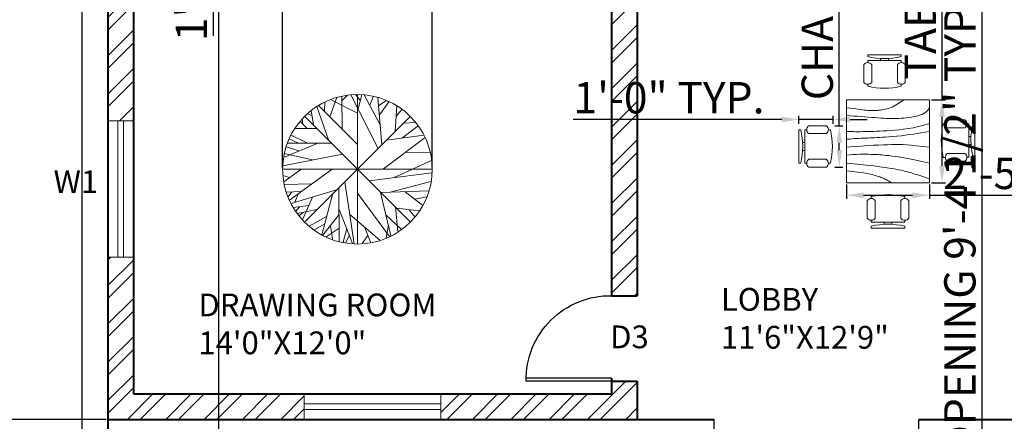
# Model space of a CAD drawing. Units: inches. Extents: x 2069 to 3028, y 691 to 1726.
# Tile 3 of 10: x 2267 to 2613, y 903 to 1044. Entities that reach past the tile are written whole.
import ezdxf

# ---------------------------------------------------------------- set-up
doc = ezdxf.new("R2010")
doc.units = ezdxf.units.IN
for name, color, linetype, lineweight in [('A-ANNO-DIMS', 2, 'Continuous', 18), ('A-DOOR', 3, 'Continuous', 25), ('A-FLOR', 7, 'Continuous', 25), ('A-FURN', 8, 'Continuous', 18), ('A-GLAZ', 4, 'Continuous', 20), ('A-WALL', 7, 'Continuous', 40)]:
    doc.layers.add(name, color=color, linetype=linetype, lineweight=lineweight)
for name, color, linetype, lineweight, true_color in [('A-ANNO-TEXT', 11, 'Continuous', 18, 0xf27172), ('A-AREA-IDEN', 11, 'Continuous', 25, 0xf27172), ('A-WALL-PATT', 143, 'Continuous', 13, 0x7aafdf), ('L-PLNT', 2, 'Continuous', 13, 0xf1eb1f)]:
    doc.layers.add(name, color=color, linetype=linetype, lineweight=lineweight, true_color=true_color)
doc.styles.get("Standard").update_dxf_attribs({"font": 'arial.ttf'})
doc.dimstyles.new('ISO-25', dxfattribs={"dimtxt": 11, "dimasz": 6, "dimexe": 1.25, "dimexo": 0.625, "dimtad": 1, "dimlunit": 3, "dimtxsty": 'Standard', "dimcen": 2.5, "dimclrd": 3, "dimclre": 5, "dimclrt": 6, "dimadec": 0, "dimazin": 0, "dimtfac": 1, "dimtmove": 0, "dimatfit": 3, "dimfxl": 1, "dimarcsym": 0})

# ---------------------------------------------------------------- blocks, each defined once
blk = doc.blocks.new('Table - Square Woodgrain 42 x 42 in.')
blk.add_line((0, -42), (42, -42))
for points in [[(0, -4), (1.704, -4.2172), (3.2358, -4.4188), (4.615, -4.604), (5.8615, -4.7721), (6.9951, -4.9224), (8.0357, -5.0541), (9.0031, -5.1667), (9.9171, -5.2594), (10.7951, -5.3316), (11.6445, -5.3836), (12.4702, -5.4157), (13.277, -5.4283), (14.0698, -5.4217), (14.8535, -5.3964), (15.6331, -5.3526), (16.4133, -5.2908), (17.1986, -5.2103), (17.9913, -5.1062), (18.793, -4.9727), (19.6056, -4.8038), (20.4307, -4.5937), (21.2701, -4.3365), (22.1256, -4.0262), (22.9989, -3.6571), (23.888, -3.2272), (24.7756, -2.7516), (25.6408, -2.2491), (26.4624, -1.7387), (27.2195, -1.2395), (27.891, -0.7703), (28.456, -0.3501), (28.8934, 0.002)], [(0, -42), (0, 0), (42, 0), (42, -42)], [(0, -8), (1.8203, -8.1001), (3.6741, -8.2149), (5.5411, -8.3408), (7.4011, -8.4741), (9.2339, -8.6112), (11.0193, -8.7484), (12.7371, -8.8821), (14.3671, -9.0086), (15.8954, -9.1246), (17.3337, -9.2278), (18.6997, -9.3159), (20.0116, -9.387), (21.2871, -9.4389), (22.5442, -9.4696), (23.8008, -9.477), (25.0749, -9.459), (26.3791, -9.4137), (27.7049, -9.3403), (29.0383, -9.2382), (30.3655, -9.1068), (31.6728, -8.9455), (32.9461, -8.7535), (34.1717, -8.5304), (35.3358, -8.2756), (36.4268, -7.9863), (37.443, -7.6521), (38.3849, -7.2603), (39.253, -6.7986), (40.048, -6.2542), (40.7705, -5.6147), (41.421, -4.8674), (42, -4)], [(42, -12), (39.1784, -12.8621), (36.4519, -13.5654), (33.8246, -14.1294), (31.3004, -14.5731), (28.8832, -14.9161), (26.577, -15.1775), (24.3858, -15.3768), (22.3136, -15.5332), (20.3622, -15.6632), (18.5254, -15.7718), (16.7947, -15.8612), (15.1618, -15.9338), (13.6183, -15.9916), (12.1558, -16.0369), (10.7659, -16.0718), (9.4403, -16.0987), (8.1703, -16.1191), (6.9461, -16.1325), (5.7577, -16.1377), (4.595, -16.1335), (3.4479, -16.1188), (2.3064, -16.0924), (1.1604, -16.0532), (0, -16)], [(42, -16), (37.6529, -16.7365), (33.8802, -17.329), (30.6179, -17.7961), (27.8015, -18.1561), (25.3668, -18.4275), (23.2497, -18.6288), (21.3859, -18.7785), (19.7111, -18.8949), (18.1693, -18.9939), (16.7375, -19.0795), (15.401, -19.1534), (14.1449, -19.217), (12.9544, -19.2717), (11.8148, -19.3191), (10.7113, -19.3606), (9.6291, -19.3976), (8.5534, -19.4323), (7.47, -19.4689), (6.3643, -19.5122), (5.222, -19.5672), (4.0288, -19.6386), (2.7703, -19.7313), (1.4321, -19.8501), (0, -20)], [(0, -24), (3.9243, -23.6805), (7.4766, -23.4138), (10.6891, -23.1954), (13.5943, -23.0205), (16.2247, -22.8847), (18.6125, -22.7832), (20.7903, -22.7116), (22.7903, -22.6651), (24.6563, -22.642), (26.4764, -22.6507), (28.35, -22.7024), (30.3766, -22.8084), (32.6555, -22.98), (35.2861, -23.2283), (38.3678, -23.5645), (42, -24)], [(42, -32), (37.392, -31.017), (33.4585, -30.2231), (30.1291, -29.5949), (27.3334, -29.109), (25.0009, -28.742), (23.0612, -28.4707), (21.4439, -28.2716), (20.0786, -28.1215), (18.8998, -28.0002), (17.8609, -27.9014), (16.9206, -27.8219), (16.0371, -27.7588), (15.1691, -27.709), (14.2748, -27.6693), (13.3128, -27.6368), (12.2415, -27.6083), (11.0295, -27.5824), (9.6867, -27.5643), (8.233, -27.5608), (6.6884, -27.5787), (5.0728, -27.6248), (3.4062, -27.7058), (1.7086, -27.8286), (0, -28)], [(0, -32), (5.4026, -32.5358), (9.9494, -33.019), (13.7424, -33.4553), (16.8834, -33.8505), (19.4743, -34.2106), (21.6171, -34.5413), (23.4136, -34.8486), (24.9657, -35.1382), (26.3614, -35.4156), (27.6332, -35.6841), (28.7995, -35.9467), (29.8788, -36.2064), (30.8897, -36.4661), (31.8507, -36.7288), (32.7802, -36.9973), (33.6968, -37.2747), (34.6175, -37.5635), (35.5531, -37.8651), (36.5128, -38.1805), (37.506, -38.5108), (38.5421, -38.8568), (39.6302, -39.2197), (40.7797, -39.6004), (42, -40)], [(0, -36), (3.0098, -36.2857), (5.5354, -36.5643), (7.6368, -36.8359), (9.374, -37.1009), (10.807, -37.3597), (11.9957, -37.6126), (13.0002, -37.8599), (13.8804, -38.102), (14.6874, -38.3393), (15.4365, -38.5729), (16.1338, -38.8041), (16.7858, -39.0341), (17.3987, -39.264), (17.9787, -39.4952), (18.5322, -39.7288), (19.0655, -39.9662), (19.5832, -40.2081), (20.0842, -40.4544), (20.5657, -40.7046), (21.0249, -40.9581), (21.459, -41.2144), (21.8653, -41.4731), (22.2409, -41.7335), (22.5831, -41.9951)]]:
    blk.add_lwpolyline(points)
blk = doc.blocks.new('Chair - Desk')
for p, q in [((-8.5, 0), (-8.5, -1)), ((-8.5, 0), (8.5, 0)), ((8.5, 0), (8.5, -1)), ((-8.5, -3), (-8.5, -4)), ((-8.5, -3), (8.5, -3)), ((-2, -3), (-2, -1.9355)), ((2, -1.9576), (2, -3)), ((8.5, -3), (8.5, -4)), ((-10.5, -5), (-10.5, -14)), ((-6.5, -14), (-6.5, -5)), ((6.5, -5), (6.5, -14)), ((10.5, -14), (10.5, -5)), ((-8.5, -15), (-8.5, -16)), ((8.5, -15), (8.5, -16))]:
    blk.add_line(p, q)
for centre, radius, start, end in [((-8.5, -6.5), 2.5, 36.8699, 143.1301), ((0, 34.625), 36.625, 256.5803, 283.4197), ((8.5, -6.5), 2.5, 36.8699, 143.1301), ((-8.5, -12.5), 2.5, 216.8699, 323.1301), ((8.5, -12.5), 2.5, 216.8699, 323.1301), ((0, 19.625), 36.625, 256.5803, 283.4197)]:
    blk.add_arc(centre, radius, start, end)
blk = doc.blocks.new('*U15')
for p, q in [((-559.96332, 1068.71262), (-421.33774, 1464.27444)), ((-537.60624, 1418.42744), (-0.98552, 1143.23876)), ((-318.48552, 1395.49124), (-202.21702, 1510.14684)), ((-314.01258, 816.46522), (-318.48552, 1492.95104)), ((-135.1407, 1515.88724), (419.3667, 426.62602)), ((61.6204, 1395.49124), (-36.75888, 1521.60224)), ((0, 1523.98984), (0, -1524)), ((12.43076, 1234.96832), (92.92336, 1515.88724)), ((464.08594, 902.45692), (137.6426, 1515.88724)), ((249.43562, 1309.49446), (325.45782, 1487.21064)), ((499.8593, 495.41938), (414.89376, 1464.27444)), ((-828.27368, 1280.83056), (-591.26628, 598.61196)), ((-792.50032, 1298.0289), (-5.45846, 512.61772)), ((-671.75888, 1183.37076), (-667.28848, 1366.81464)), ((432.78298, 1298.0289), (589.29524, 1401.23164)), ((450.66966, 1108.84208), (647.43076, 1378.29544)), ((803.94302, 1292.29612), (768.16966, 776.33322)), ((790.52928, 1080.17818), (911.26818, 1223.50022)), ((-1114.47072, 925.38804), (-1127.887, 1022.84784)), ((1066.8, 1066.8), (-1066.8, -1066.8)), ((1066.8, -1066.8), (-1066.8, 1066.8)), ((-1020.56438, 1131.7732), (-926.6555, 1097.37652)), ((-940.07178, 1194.83632), (-895.35, 902.45692)), ((-1266.51258, 833.66356), (-832.74662, 833.66356)), ((-1163.66036, 971.25282), (-1029.50772, 839.39634)), ((920.21152, 638.74396), (1242.18446, 890.99136)), ((942.57114, 942.58892), (1184.04894, 954.05448)), ((-1391.72442, 621.54308), (-1212.85, 535.55138)), ((-1351.47812, 696.07176), (-1020.56438, 529.8186)), ((1380.81004, 644.47674), (531.16226, 8.12292)), ((593.76818, 592.87918), (1353.98002, 696.07176)), ((-819.33034, 524.08582), (-1503.51998, 237.4392)), ((-1449.8574, 455.28992), (-1194.96332, 375.02846)), ((-1423.02738, 529.8186), (-528.66036, 529.8186)), ((-1516.93626, 71.1835), (-305.06924, 306.2351)), ((-1490.10624, 323.43344), (-913.23922, 191.57696)), ((978.3445, 340.63178), (1479.19186, 346.36456)), ((-1387.25148, -628.2309), (-515.24662, 2.39014)), ((745.81004, -169.59834), (1510.49228, 180.1114)), ((-1524, 0), (1524, 0)), ((-1516.93626, -123.73356), (-1378.30814, -169.59834)), ((-1150.24662, -3.34264), (-1499.04958, -255.59258)), ((236.02188, -232.65892), (1514.96522, -72.13854)), ((-1485.6333, -312.92038), (-926.6555, -295.72204)), ((-376.6185, -381.71628), (-372.1481, -1465.2371)), ((-255.8796, -255.59258), (-63.59144, -1516.83212)), ((669.79038, -467.71052), (1497.07854, -249.85726)), ((-1449.8574, -467.71052), (-1150.24662, -456.24496)), ((-1338.06438, -461.9752), (-1409.61364, -559.43754)), ((-1351.47812, -697.0268), (-425.80814, -421.84574)), ((-1199.43626, -490.64164), (-1275.45592, -668.3629)), ((-913.23922, -570.9031), (-1118.94366, -1029.53566)), ((-506.30074, -513.57276), (-725.42146, -1339.1134)), ((-0.98552, -484.90886), (656.3741, -1367.7773)), ((473.02928, -473.44076), (678.73372, -1356.31174)), ((477.49968, -473.44076), (1456.83224, -439.04662)), ((969.40116, -461.9752), (1331.6204, -737.15626)), ((1166.16226, -611.03256), (1412.113, -565.17032)), ((-989.25888, -737.15626), (-1306.75888, -777.28572)), ((-1181.54958, -765.82016), (-1257.56924, -851.8144)), ((772.6426, -765.82016), (821.83224, -1270.3175)), ((799.47262, -794.4866), (1260.07114, -846.08162)), ((-823.80074, -823.1505), (-1221.79334, -903.41196)), ((-1110.00032, -880.4783), (-1186.01998, -949.2742)), ((-627.04218, -960.73976), (-984.78848, -1161.39214)), ((-372.1481, -920.6103), (-703.06438, -1344.84618)), ((-372.1481, -817.41772), (-99.3648, -1511.10188)), ((-157.50032, -920.6103), (455.1426, -1448.03876)), ((580.3519, -926.34308), (897.8519, -1230.18804)), ((1054.3667, -828.88328), (1170.6352, -966.47254)), ((-667.28848, -1115.5299), (-881.93626, -1235.92082)), ((-372.1481, -1201.52414), (-635.98552, -1379.24286)), ((-546.54958, -1155.65936), (-506.30074, -1425.1051)), ((151.05634, -1184.32326), (267.32484, -1488.16822)), ((629.54408, -1138.46102), (584.82484, -1396.4412)), ((-215.6333, -1207.25692), (-291.6555, -1488.16822)), ((-161.97072, -1339.1134), (-237.99292, -1493.901)), ((213.66226, -1350.57896), (97.39376, -1511.10188))]:
    blk.add_line(p, q)
blk.add_circle((0, 0), 1524)
blk = doc.blocks.new('DOOR-SWING-30IN')
for p, q in [((-1, 0), (-1, 30)), ((0, 0), (0, 30))]:
    blk.add_line(p, q)
blk.add_arc((-0.5, 0.5), 29.5, 89.029, 180.971)
blk = doc.blocks.new('WINDOW-SASH-48IN')
for p, q in [((0, 0), (48, 0)), ((0, -2), (48, -2))]:
    blk.add_line(p, q)
blk = doc.blocks.new('*D46')
at = {"layer": 'A-ANNO-DIMS', "color": 3, "lineweight": -2, "transparency": 16777216}
for p, q in [((2554.97, 1007.13), (2554.97, 1159.02)), ((2554.97, 998.55), (2554.97, 1001.13))]:
    blk.add_line(p, q, dxfattribs=at)
at = {"layer": 'A-ANNO-DIMS', "color": 5, "lineweight": -2, "transparency": 16777216}
for p, q in [((2553.4, 1007.13), (2556.22, 1007.13)), ((2553.4, 992.55), (2556.22, 992.55))]:
    blk.add_line(p, q, dxfattribs=at)
at = {"layer": 'A-ANNO-DIMS', "color": 3, "transparency": 16777216}
for points in [[(2553.97, 1001.13), (2555.97, 1001.13), (2554.97, 1007.13)], [(2553.97, 998.55), (2555.97, 998.55), (2554.97, 992.55)]]:
    blk.add_solid(points, dxfattribs=at)
at = {"layer": 'Defpoints', "color": 0, "transparency": 16777216}
for p in [(2552.78, 1007.13), (2554.97, 1007.13), (2552.78, 992.55)]:
    blk.add_point(p, dxfattribs=at)
at = {"layer": 'A-ANNO-DIMS', "color": 6, "transparency": 16777216, "insert": (2548.65, 1086.08), "char_height": 11, "attachment_point": 5, "rotation": 90}
blk.add_mtext('CHAIR 1\'-2 1/2" TYP.', dxfattribs=at)
blk = doc.blocks.new('*D47')
at = {"layer": 'A-ANNO-DIMS', "color": 5, "lineweight": -2, "transparency": 16777216}
for p, q in [((2540.74, 1007.76), (2540.74, 1010.57)), ((2552.78, 1007.76), (2552.78, 1010.57))]:
    blk.add_line(p, q, dxfattribs=at)
at = {"layer": 'A-ANNO-DIMS', "color": 3, "lineweight": -2, "transparency": 16777216}
for p, q in [((2534.74, 1009.32), (2461.47, 1009.32)), ((2552.78, 1009.32), (2540.74, 1009.32)), ((2558.78, 1009.32), (2564.78, 1009.32))]:
    blk.add_line(p, q, dxfattribs=at)
at = {"layer": 'A-ANNO-DIMS', "color": 3, "transparency": 16777216}
for points in [[(2534.74, 1010.32), (2534.74, 1008.32), (2540.74, 1009.32)], [(2558.78, 1010.32), (2558.78, 1008.32), (2552.78, 1009.32)]]:
    blk.add_solid(points, dxfattribs=at)
at = {"layer": 'Defpoints', "color": 0, "transparency": 16777216}
for p in [(2540.74, 1009.32), (2540.74, 1007.13), (2552.78, 1007.13)]:
    blk.add_point(p, dxfattribs=at)
at = {"layer": 'A-ANNO-DIMS', "color": 6, "transparency": 16777216, "insert": (2495.11, 1015.56), "char_height": 11, "attachment_point": 5}
blk.add_mtext('1\'-0" TYP.', dxfattribs=at)
blk = doc.blocks.new('*D66')
at = {"layer": 'A-ANNO-DIMS', "color": 3, "lineweight": -2, "transparency": 16777216}
for p, q in [((2591.06, 1016.25), (2591.06, 1105.97)), ((2591.06, 993.08), (2591.06, 1010.25))]:
    blk.add_line(p, q, dxfattribs=at)
at = {"layer": 'A-ANNO-DIMS', "color": 5, "lineweight": -2, "transparency": 16777216}
for p, q in [((2587.31, 1016.25), (2592.31, 1016.25)), ((2587.31, 987.08), (2592.31, 987.08))]:
    blk.add_line(p, q, dxfattribs=at)
at = {"layer": 'A-ANNO-DIMS', "color": 3, "transparency": 16777216}
for points in [[(2590.06, 1010.25), (2592.06, 1010.25), (2591.06, 1016.25)], [(2590.06, 993.08), (2592.06, 993.08), (2591.06, 987.08)]]:
    blk.add_solid(points, dxfattribs=at)
at = {"layer": 'Defpoints', "color": 0, "transparency": 16777216}
for p in [(2586.69, 1016.25), (2591.06, 1016.25), (2586.69, 987.08)]:
    blk.add_point(p, dxfattribs=at)
at = {"layer": 'A-ANNO-DIMS', "color": 6, "transparency": 16777216, "insert": (2584.82, 1064.11), "char_height": 11, "attachment_point": 5, "rotation": 90}
blk.add_mtext('TABLE 2\'-5"', dxfattribs=at)
blk = doc.blocks.new('*D67')
at = {"layer": 'A-ANNO-DIMS', "color": 5, "lineweight": -2, "transparency": 16777216}
for p, q in [((2557.52, 986.45), (2557.52, 981.45)), ((2586.69, 986.45), (2586.69, 981.45))]:
    blk.add_line(p, q, dxfattribs=at)
at = {"layer": 'A-ANNO-DIMS', "color": 3, "lineweight": -2, "transparency": 16777216}
for p, q in [((2563.52, 982.7), (2580.69, 982.7)), ((2586.69, 982.7), (2623.36, 982.7))]:
    blk.add_line(p, q, dxfattribs=at)
at = {"layer": 'A-ANNO-DIMS', "color": 3, "transparency": 16777216}
for points in [[(2563.52, 983.7), (2563.52, 981.7), (2557.52, 982.7)], [(2580.69, 983.7), (2580.69, 981.7), (2586.69, 982.7)]]:
    blk.add_solid(points, dxfattribs=at)
at = {"layer": 'Defpoints', "color": 0, "transparency": 16777216}
for p in [(2557.52, 987.08), (2586.69, 987.08), (2586.69, 982.7)]:
    blk.add_point(p, dxfattribs=at)
at = {"layer": 'A-ANNO-DIMS', "color": 6, "transparency": 16777216, "insert": (2608.03, 988.95), "char_height": 11, "attachment_point": 5}
blk.add_mtext('2\'-5"', dxfattribs=at)
blk = doc.blocks.new('*D72')
at = {"layer": 'A-ANNO-DIMS', "color": 5, "lineweight": -2, "transparency": 16777216}
for p, q in [((2621.33, 1178.39), (2603.83, 1178.39)), ((2621.33, 1065.89), (2603.83, 1065.89))]:
    blk.add_line(p, q, dxfattribs=at)
at = {"layer": 'A-ANNO-DIMS', "color": 3, "lineweight": -2, "transparency": 16777216}
for p, q in [((2605.08, 1172.39), (2605.08, 1071.89)), ((2605.08, 1065.89), (2605.08, 833.73))]:
    blk.add_line(p, q, dxfattribs=at)
at = {"layer": 'A-ANNO-DIMS', "color": 3, "transparency": 16777216}
for points in [[(2604.08, 1172.39), (2606.08, 1172.39), (2605.08, 1178.39)], [(2604.08, 1071.89), (2606.08, 1071.89), (2605.08, 1065.89)]]:
    blk.add_solid(points, dxfattribs=at)
at = {"layer": 'Defpoints', "color": 0, "transparency": 16777216}
for p in [(2621.95, 1178.39), (2605.08, 1065.89), (2621.95, 1065.89)]:
    blk.add_point(p, dxfattribs=at)
at = {"layer": 'A-ANNO-DIMS', "color": 6, "transparency": 16777216, "insert": (2598.76, 946.81), "char_height": 11, "attachment_point": 5, "rotation": 90}
blk.add_mtext('CASED OPENING 9\'-4 1/2" TYP.', dxfattribs=at)
blk = doc.blocks.new('*D85')
at = {"layer": 'A-ANNO-DIMS', "color": 5, "lineweight": -2, "transparency": 16777216}
for p, q in [((2339.28, 1095.19), (2333.7, 1095.19)), ((2339.28, 1074.19), (2333.7, 1074.19))]:
    blk.add_line(p, q, dxfattribs=at)
at = {"layer": 'A-ANNO-DIMS', "color": 3, "lineweight": -2, "transparency": 16777216}
for p, q in [((2334.95, 1089.19), (2334.95, 1080.19)), ((2334.95, 1074.19), (2334.95, 1038.73))]:
    blk.add_line(p, q, dxfattribs=at)
at = {"layer": 'A-ANNO-DIMS', "color": 3, "transparency": 16777216}
for points in [[(2333.95, 1089.19), (2335.95, 1089.19), (2334.95, 1095.19)], [(2333.95, 1080.19), (2335.95, 1080.19), (2334.95, 1074.19)]]:
    blk.add_solid(points, dxfattribs=at)
at = {"layer": 'Defpoints', "color": 0, "transparency": 16777216}
for p in [(2339.91, 1095.19), (2334.95, 1074.19), (2339.91, 1074.19)]:
    blk.add_point(p, dxfattribs=at)
at = {"layer": 'A-ANNO-DIMS', "color": 6, "transparency": 16777216, "insert": (2328.71, 1053.46), "char_height": 11, "attachment_point": 5, "rotation": 90}
blk.add_mtext('1\'-9"', dxfattribs=at)
blk = doc.blocks.new('*D87')
at = {"layer": 'A-ANNO-DIMS', "color": 5, "lineweight": -2, "transparency": 16777216}
for p, q in [((2297.33, 1487.39), (2090.2, 1487.39)), ((2297.33, 903.89), (2090.2, 903.89))]:
    blk.add_line(p, q, dxfattribs=at)
at = {"layer": 'A-ANNO-DIMS', "color": 3, "lineweight": -2, "transparency": 16777216}
blk.add_line((2091.45, 909.89), (2091.45, 1481.39), dxfattribs=at)
at = {"layer": 'A-ANNO-DIMS', "color": 3, "transparency": 16777216}
for points in [[(2090.45, 1481.39), (2092.45, 1481.39), (2091.45, 1487.39)], [(2090.45, 909.89), (2092.45, 909.89), (2091.45, 903.89)]]:
    blk.add_solid(points, dxfattribs=at)
at = {"layer": 'Defpoints', "color": 0, "transparency": 16777216}
for p in [(2091.45, 1487.39), (2297.95, 1487.39), (2297.95, 903.89)]:
    blk.add_point(p, dxfattribs=at)
at = {"layer": 'A-ANNO-DIMS', "color": 6, "transparency": 16777216, "insert": (2085.14, 1195.64), "char_height": 11, "attachment_point": 5, "rotation": 90}
blk.add_mtext('48\'-7 1/2"', dxfattribs=at)
blk = doc.blocks.new('*D88')
at = {"layer": 'A-ANNO-DIMS', "color": 5, "lineweight": -2, "transparency": 16777216}
for p, q in [((2288.92, 738.01), (2288.92, 1704.14)), ((2336.92, 738.01), (2336.92, 1704.14))]:
    blk.add_line(p, q, dxfattribs=at)
at = {"layer": 'A-ANNO-DIMS', "color": 3, "lineweight": -2, "transparency": 16777216}
blk.add_line((2294.92, 1702.89), (2330.92, 1702.89), dxfattribs=at)
at = {"layer": 'A-ANNO-DIMS', "color": 3, "transparency": 16777216}
for points in [[(2294.92, 1703.89), (2294.92, 1701.89), (2288.92, 1702.89)], [(2330.92, 1703.89), (2330.92, 1701.89), (2336.92, 1702.89)]]:
    blk.add_solid(points, dxfattribs=at)
at = {"layer": 'Defpoints', "color": 0, "transparency": 16777216}
for p in [(2336.92, 1702.89), (2288.92, 737.39), (2336.92, 737.39)]:
    blk.add_point(p, dxfattribs=at)
at = {"layer": 'A-ANNO-DIMS', "color": 6, "transparency": 16777216, "insert": (2312.92, 1709.13), "char_height": 11, "attachment_point": 5}
blk.add_mtext('4\'-0"', dxfattribs=at)
blk = doc.blocks.new('*D89')
at = {"layer": 'A-ANNO-DIMS', "color": 5, "lineweight": -2, "transparency": 16777216}
for p, q in [((2336.92, 747.01), (2336.92, 1704.14)), ((2711.95, 747.01), (2711.95, 1704.14))]:
    blk.add_line(p, q, dxfattribs=at)
at = {"layer": 'A-ANNO-DIMS', "color": 3, "lineweight": -2, "transparency": 16777216}
blk.add_line((2342.92, 1702.89), (2705.95, 1702.89), dxfattribs=at)
at = {"layer": 'A-ANNO-DIMS', "color": 3, "transparency": 16777216}
for points in [[(2342.92, 1703.89), (2342.92, 1701.89), (2336.92, 1702.89)], [(2705.95, 1703.89), (2705.95, 1701.89), (2711.95, 1702.89)]]:
    blk.add_solid(points, dxfattribs=at)
at = {"layer": 'Defpoints', "color": 0, "transparency": 16777216}
for p in [(2711.95, 1702.89), (2336.92, 746.39), (2711.95, 746.39)]:
    blk.add_point(p, dxfattribs=at)
at = {"layer": 'A-ANNO-DIMS', "color": 6, "transparency": 16777216, "insert": (2524.44, 1709.13), "char_height": 11, "attachment_point": 5}
blk.add_mtext('31\'-3"', dxfattribs=at)
blk = doc.blocks.new('*D92')
at = {"layer": 'A-ANNO-DIMS', "color": 5, "lineweight": -2, "transparency": 16777216}
for p, q in [((2359.37, 992.45), (2359.37, 1704.14)), ((2411.94, 992.45), (2411.94, 1704.14))]:
    blk.add_line(p, q, dxfattribs=at)
at = {"layer": 'A-ANNO-DIMS', "color": 3, "lineweight": -2, "transparency": 16777216}
for p, q in [((2365.37, 1702.89), (2405.94, 1702.89)), ((2411.94, 1702.89), (2474.5, 1702.89))]:
    blk.add_line(p, q, dxfattribs=at)
at = {"layer": 'A-ANNO-DIMS', "color": 3, "transparency": 16777216}
for points in [[(2365.37, 1703.89), (2365.37, 1701.89), (2359.37, 1702.89)], [(2405.94, 1703.89), (2405.94, 1701.89), (2411.94, 1702.89)]]:
    blk.add_solid(points, dxfattribs=at)
at = {"layer": 'Defpoints', "color": 0, "transparency": 16777216}
for p in [(2411.94, 1702.89), (2359.37, 991.83), (2411.94, 991.83)]:
    blk.add_point(p, dxfattribs=at)
at = {"layer": 'A-ANNO-DIMS', "color": 6, "transparency": 16777216, "insert": (2446.22, 1709.2), "char_height": 11, "attachment_point": 5}
blk.add_mtext('4\'-4 1/2"', dxfattribs=at)

msp = doc.modelspace()

# ---------------------------------------------------------------- hatches: boundary and pattern name
at = {"layer": 'A-WALL-PATT'}
h = msp.add_hatch(dxfattribs=at)
h.set_pattern_fill('ANSI32', color=256)
h.paths.add_polyline_path([(2675.951, 1487.387), (2576.951, 1487.387), (2576.951, 1478.387), (2621.951, 1478.387), (2621.951, 1365.287), (2630.951, 1365.287), (2630.951, 1478.387), (2675.951, 1478.387)])
h.paths.add_polyline_path([(2765.951, 1487.387), (2711.951, 1487.387), (2711.951, 1478.387), (2756.951, 1478.387), (2756.951, 1424.387), (2765.951, 1424.387)])
h.paths.add_polyline_path([(2528.951, 1487.387), (2407.751, 1487.387), (2407.751, 1478.387), (2474.951, 1478.387), (2474.951, 1434.887), (2498.951, 1434.887), (2498.951, 1374.887), (2474.951, 1374.887), (2474.951, 1365.287), (2483.951, 1365.287), (2483.951, 1370.387), (2507.951, 1370.387), (2507.951, 1439.387), (2483.951, 1439.387), (2483.951, 1478.387), (2528.951, 1478.387)])
h.paths.add_polyline_path([(2374.151, 1487.387), (2297.951, 1487.387), (2297.951, 1424.387), (2306.951, 1424.387), (2306.951, 1478.387), (2374.151, 1478.387)])
h.paths.add_polyline_path([(2507.951, 1334.387), (2483.951, 1334.387), (2483.951, 1338.887), (2474.951, 1338.887), (2474.951, 1334.387), (2306.951, 1334.387), (2306.951, 1388.387), (2297.951, 1388.387), (2297.951, 1334.387), (2267.951, 1334.387), (2267.951, 1274.387), (2276.951, 1274.387), (2276.951, 1325.387), (2297.951, 1325.387), (2423.951, 1325.387), (2423.951, 1187.387), (2419.451, 1187.387), (2419.451, 1178.387), (2432.951, 1178.387), (2432.951, 1325.387), (2507.951, 1325.387)])
h.paths.add_polyline_path([(2795.951, 1334.387), (2630.951, 1334.387), (2630.951, 1338.887), (2621.951, 1338.887), (2621.951, 1178.387), (2635.451, 1178.387), (2635.451, 1187.387), (2630.951, 1187.387), (2630.951, 1325.387), (2786.951, 1325.387), (2786.951, 1274.387), (2795.951, 1274.387)])
h.paths.add_polyline_path([(2765.951, 1388.387), (2756.951, 1388.387), (2756.951, 1334.387), (2765.951, 1334.387)])
h.paths.add_polyline_path([(2795.951, 1238.387), (2786.951, 1238.387), (2786.951, 1187.387), (2665.451, 1187.387), (2665.451, 1178.387), (2795.951, 1178.387)], flags=17)
h.paths.add_polyline_path([(2389.451, 1187.387), (2276.951, 1187.387), (2276.951, 1238.387), (2267.951, 1238.387), (2267.951, 1178.387), (2297.951, 1178.387), (2297.951, 1173.287), (2307.451, 1173.287), (2307.451, 1178.387), (2389.451, 1178.387)])
h.paths.add_polyline_path([(2377.451, 1142.387), (2306.951, 1142.387), (2306.951, 1146.887), (2297.951, 1146.887), (2297.951, 1142.387), (2297.951, 1137.887), (2306.951, 1137.887), (2372.951, 1137.887), (2372.951, 1133.387), (2377.451, 1133.387)])
h.paths.add_polyline_path([(2795.951, 1065.887), (2665.451, 1065.887), (2665.451, 1056.887), (2786.951, 1056.887), (2786.951, 1002.887), (2795.951, 1002.887), (2795.951, 1056.887)])
h.paths.add_polyline_path([(2795.951, 966.887), (2786.951, 966.887), (2786.951, 912.887), (2732.951, 912.887), (2732.951, 903.887), (2795.951, 903.887)])
h.paths.add_polyline_path([(2483.951, 917.387), (2474.951, 917.387), (2474.951, 912.887), (2414.951, 912.887), (2414.951, 903.887), (2483.951, 903.887)])
h.paths.add_polyline_path([(2366.951, 912.887), (2306.951, 912.887), (2306.951, 960.887), (2297.951, 960.887), (2297.951, 903.887), (2366.951, 903.887)])
h.paths.add_polyline_path([(2498.951, 1056.887), (2498.951, 1065.887), (2377.451, 1065.887), (2377.451, 1111.787), (2372.951, 1111.787), (2372.951, 1065.887), (2306.951, 1065.887), (2306.951, 1116.287), (2297.951, 1116.287), (2297.951, 1056.887), (2297.951, 1008.887), (2306.951, 1008.887), (2306.951, 1056.887), (2474.951, 1056.887), (2474.951, 947.387), (2483.951, 947.387), (2483.951, 1056.887)])

# ---------------------------------------------------------------- linework, layer by layer
at = {"layer": 'A-FLOR'}
for p, q in [((2510.951, 867.887), (2510.951, 903.887)), ((2582.951, 867.887), (2582.951, 903.887))]:
    msp.add_line(p, q, dxfattribs=at)
at = {"layer": 'A-GLAZ'}
for p, q in [((2306.951, 1008.887), (2297.951, 1008.887)), ((2306.951, 960.887), (2297.951, 960.887)), ((2366.951, 912.887), (2366.951, 903.887)), ((2414.951, 912.887), (2414.951, 903.887))]:
    msp.add_line(p, q, dxfattribs=at)
at = {"layer": 'A-WALL'}
for p, q in [((2297.951, 1056.887), (2297.951, 867.887)), ((2306.951, 1056.887), (2306.951, 912.887)), ((2474.951, 1056.887), (2474.951, 947.387)), ((2483.951, 1056.887), (2483.951, 947.387)), ((2474.951, 947.387), (2483.951, 947.387)), ((2474.951, 918.387), (2474.951, 912.887)), ((2474.951, 917.387), (2483.951, 917.387)), ((2483.951, 917.387), (2483.951, 903.887)), ((2306.951, 912.887), (2474.951, 912.887)), ((2297.951, 903.887), (2510.951, 903.887)), ((2582.951, 903.887), (2795.951, 903.887))]:
    msp.add_line(p, q, dxfattribs=at)

# ---------------------------------------------------------------- block references
at = {"layer": 'A-DOOR', "extrusion": (0, 0, -1), "zscale": -1, "rotation": 269.9999999999995}
msp.add_blockref('DOOR-SWING-30IN', (-2474.951, 917.387), dxfattribs=at)
at = {"layer": 'A-FURN', "xscale": 0.6944950846218003, "yscale": 0.6944950846218003, "zscale": 0.6944950846218003}
for name, p in [('Chair - Desk', (2570.862, 1032.109)), ('Table - Square Woodgrain 42 x 42 in.', (2557.517, 1016.248))]:
    msp.add_blockref(name, p, dxfattribs=at)
at = {"layer": 'A-FURN'}
for p, xscale, yscale, zscale, rotation in [((2540.74, 999.843), 0.6944950846218003, 0.6944950846218003, 0.6944950846218003, 90), ((2602.597, 1001.941), 0.6944950846218008, 0.6944950846218008, 0.6944950846218008, 270.1537049626395), ((2572.089, 971.127), 0.6944950846218003, 0.6944950846218003, 0.6944950846218003, 180)]:
    msp.add_blockref('Chair - Desk', p, dxfattribs=dict(at, xscale=xscale, yscale=yscale, zscale=zscale, rotation=rotation))
at = {"layer": 'A-GLAZ', "rotation": 269.9999999999987}
msp.add_blockref('WINDOW-SASH-48IN', (2303.451, 1008.887), dxfattribs=at)
at = {"layer": 'A-GLAZ'}
msp.add_blockref('WINDOW-SASH-48IN', (2366.951, 909.387), dxfattribs=at)
at = {"layer": 'L-PLNT', "xscale": 0.0172476561611968, "yscale": 0.0172476561611968, "zscale": 0.0172476561611968}
msp.add_blockref('*U15', (2385.651, 991.83), dxfattribs=at)

# ---------------------------------------------------------------- texts
at = {"layer": 'A-ANNO-TEXT', "char_height": 8, "attachment_point": 1}
for s, insert in [('{\\fArial|b1|i0|c0|p34;W1}', (2278.894, 991.431)), ('{\\fArial|b1|i0|c0|p34;D3}', (2474.451, 936.911))]:
    msp.add_mtext_dynamic_manual_height_columns(s, width=34.05605, gutter_width=12.5, heights=[0], dxfattribs=dict(at, insert=insert))
at = {"layer": 'A-AREA-IDEN', "char_height": 8, "attachment_point": 1}
for s, insert in [('DRAWING ROOM\\P14\'0"X12\'0"', (2329.775, 948.143)), ('LOBBY\\P11\'6"X12\'9"', (2513.377, 950.096))]:
    msp.add_mtext_dynamic_manual_height_columns(s, width=119.20948, gutter_width=12.5, heights=[0], dxfattribs=dict(at, insert=insert))

# ---------------------------------------------------------------- dimensions: what is measured, and where the dimension line sits
at = {"layer": 'A-ANNO-DIMS'}
for base, p1, p2, picture, middle in [((2411.936, 1702.887), (2359.366, 991.83), (2411.936, 991.83), '*D92', (2446.219, 1709.199)), ((2336.919, 1702.887), (2288.919, 737.387), (2336.919, 737.387), '*D88', (2312.919, 1709.128)), ((2711.951, 1702.887), (2336.919, 746.387), (2711.951, 746.387), '*D89', (2524.435, 1709.132)), ((2586.686, 982.704), (2557.517, 987.079), (2586.686, 987.079), '*D67', (2608.025, 988.945))]:
    dim = msp.add_linear_dim(base=base, p1=p1, p2=p2, dimstyle='ISO-25', override={"dimdec": 1, "dimlfac": 1, "dimrnd": 0, "dimzin": 1, "dimdsep": 46, "dimlunit": 4, "dimfrac": 2}, dxfattribs=at)
    dim.commit()
    dim.dimension.update_dxf_attribs({"geometry": picture, "text_midpoint": middle})
for base, p1, p2, angle, picture, middle in [((2091.451, 1487.387), (2297.951, 903.887), (2297.951, 1487.387), 90, '*D87', (2085.139, 1195.637)), ((2334.948, 1074.186), (2339.905, 1095.186), (2339.905, 1074.186), 270, '*D85', (2328.707, 1053.458))]:
    dim = msp.add_linear_dim(base=base, p1=p1, p2=p2, angle=angle, dimstyle='ISO-25', override={"dimdec": 1, "dimlfac": 1, "dimrnd": 0, "dimzin": 1, "dimdsep": 46, "dimlunit": 4, "dimfrac": 2}, dxfattribs=at)
    dim.commit()
    dim.dimension.update_dxf_attribs({"geometry": picture, "text_midpoint": middle})
for base, p1, p2, angle, text, picture, middle in [((2605.076, 1065.887), (2621.951, 1178.387), (2621.951, 1065.887), 270, 'CASED OPENING <> TYP.', '*D72', (2598.76, 946.808)), ((2554.965, 1007.135), (2552.778, 992.55), (2552.778, 1007.135), 90, 'CHAIR <> TYP.', '*D46', (2548.653, 1086.078)), ((2591.061, 1016.25), (2586.686, 987.079), (2586.686, 1016.25), 90, 'TABLE <>', '*D66', (2584.82, 1064.11)), ((2540.74, 1009.322), (2552.778, 1007.135), (2540.74, 1007.135), 180, '<> TYP.', '*D47', (2495.107, 1015.564))]:
    dim = msp.add_linear_dim(base=base, p1=p1, p2=p2, angle=angle, text=text, dimstyle='ISO-25', override={"dimdec": 1, "dimlfac": 1, "dimrnd": 0, "dimzin": 1, "dimdsep": 46, "dimlunit": 4, "dimfrac": 2}, dxfattribs=at)
    dim.commit()
    dim.dimension.update_dxf_attribs({"geometry": picture, "text_midpoint": middle})

doc.saveas('drawing.dxf')
